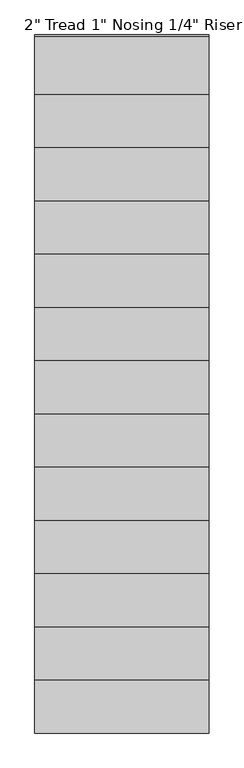
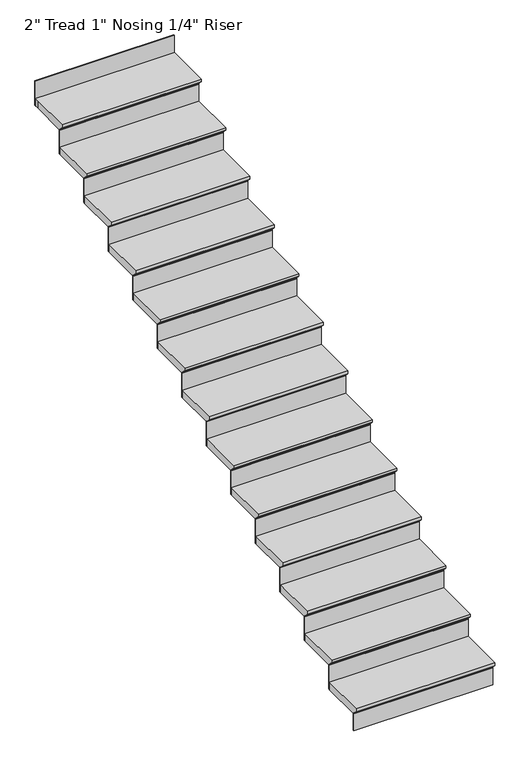
"""IFC4 building model written with IfcOpenShell, lengths in millimetres: stair flight geometry."""

from ifc_helpers import new_model, si_unit, origin, place, context, project, spatial, faceted_brep, source, transform, mapped, element, save


def stair_flight_ec606b3e(model_context):
    return source(origin(), model_context, "Body", "Brep", [
        faceted_brep([(-2703.0415084, -23154.3851539, 49768.9005799), (-2703.0415084, -23154.3851539, 49787.9505799), (-3617.4415084, -23154.3851539, 49787.9505799), (-3617.4415084, -23154.3851539, 49768.9005799), (-2703.0415084, -23128.9851539, 49743.5005799), (-3617.4415084, -23128.9851539, 49743.5005799), (-2703.0415084, -22849.5851539, 49787.9505799), (-3617.4415084, -22849.5851539, 49787.9505799), (-3617.4415084, -23128.9851539, 49737.1505799), (-3617.4415084, -22849.5851539, 49737.1505799), (-2703.0415084, -22849.5851539, 49737.1505799), (-2703.0415084, -23128.9851539, 49737.1505799)], [[[0, 1, 2, 3]], [[4, 0, 3, 5]], [[2, 1, 6, 7]], [[8, 9, 10, 11]], [[2, 7, 9, 8, 5, 3]], [[8, 11, 4, 5]], [[6, 1, 0, 4, 11, 10]], [[7, 6, 10, 9]]]),
        faceted_brep([(-2703.0415084, -23128.9851539, 49737.1505799), (-2703.0415084, -23128.9851539, 49618.6172466), (-2703.0415084, -23122.6351539, 49618.6172466), (-2703.0415084, -23122.6351539, 49737.1505799), (-3617.4415084, -23128.9851539, 49737.1505799), (-3617.4415084, -23122.6351539, 49737.1505799), (-3617.4415084, -23122.6351539, 49618.6172466), (-3617.4415084, -23128.9851539, 49618.6172466)], [[[0, 1, 2, 3]], [[4, 5, 6, 7]], [[1, 0, 4, 7]], [[2, 1, 7, 6]], [[3, 2, 6, 5]], [[0, 3, 5, 4]]]),
        faceted_brep([(-2703.0415084, -22849.5851539, 49906.4839133), (-2703.0415084, -22849.5851539, 49737.1505799), (-2703.0415084, -22843.2351539, 49737.1505799), (-2703.0415084, -22843.2351539, 49906.4839133), (-3617.4415084, -22849.5851539, 49906.4839133), (-3617.4415084, -22843.2351539, 49906.4839133), (-3617.4415084, -22843.2351539, 49737.1505799), (-3617.4415084, -22849.5851539, 49737.1505799)], [[[0, 1, 2, 3]], [[4, 5, 6, 7]], [[1, 0, 4, 7]], [[2, 1, 7, 6]], [[3, 2, 6, 5]], [[0, 3, 5, 4]]]),
        faceted_brep([(-3617.4415084, -22874.9851539, 49957.2839133), (-2703.0415084, -22874.9851539, 49957.2839133), (-2703.0415084, -22570.1851539, 49957.2839133), (-3617.4415084, -22570.1851539, 49957.2839133), (-3617.4415084, -22849.5851539, 49906.4839133), (-3617.4415084, -22570.1851539, 49906.4839133), (-2703.0415084, -22570.1851539, 49906.4839133), (-2703.0415084, -22849.5851539, 49906.4839133), (-3617.4415084, -22849.5851539, 49912.8339133), (-3617.4415084, -22874.9851539, 49938.2339133), (-2703.0415084, -22849.5851539, 49912.8339133), (-2703.0415084, -22874.9851539, 49938.2339133)], [[[0, 1, 2, 3]], [[4, 5, 6, 7]], [[0, 3, 5, 4, 8, 9]], [[4, 7, 10, 8]], [[2, 1, 11, 10, 7, 6]], [[3, 2, 6, 5]], [[11, 1, 0, 9]], [[10, 11, 9, 8]]]),
        faceted_brep([(-2703.0415084, -22570.1851539, 50075.8172466), (-2703.0415084, -22570.1851539, 49906.4839133), (-2703.0415084, -22563.8351539, 49906.4839133), (-2703.0415084, -22563.8351539, 50075.8172466), (-3617.4415084, -22570.1851539, 50075.8172466), (-3617.4415084, -22563.8351539, 50075.8172466), (-3617.4415084, -22563.8351539, 49906.4839133), (-3617.4415084, -22570.1851539, 49906.4839133)], [[[0, 1, 2, 3]], [[4, 5, 6, 7]], [[1, 0, 4, 7]], [[2, 1, 7, 6]], [[3, 2, 6, 5]], [[0, 3, 5, 4]]]),
        faceted_brep([(-3617.4415084, -22595.5851539, 50126.6172466), (-2703.0415084, -22595.5851539, 50126.6172466), (-2703.0415084, -22290.7851539, 50126.6172466), (-3617.4415084, -22290.7851539, 50126.6172466), (-3617.4415084, -22570.1851539, 50075.8172466), (-3617.4415084, -22290.7851539, 50075.8172466), (-2703.0415084, -22290.7851539, 50075.8172466), (-2703.0415084, -22570.1851539, 50075.8172466), (-3617.4415084, -22570.1851539, 50082.1672466), (-3617.4415084, -22595.5851539, 50107.5672466), (-2703.0415084, -22570.1851539, 50082.1672466), (-2703.0415084, -22595.5851539, 50107.5672466)], [[[0, 1, 2, 3]], [[4, 5, 6, 7]], [[0, 3, 5, 4, 8, 9]], [[4, 7, 10, 8]], [[2, 1, 11, 10, 7, 6]], [[3, 2, 6, 5]], [[11, 1, 0, 9]], [[10, 11, 9, 8]]]),
        faceted_brep([(-2703.0415084, -22290.7851539, 50245.1505799), (-2703.0415084, -22290.7851539, 50075.8172466), (-2703.0415084, -22284.4351539, 50075.8172466), (-2703.0415084, -22284.4351539, 50245.1505799), (-3617.4415084, -22290.7851539, 50245.1505799), (-3617.4415084, -22284.4351539, 50245.1505799), (-3617.4415084, -22284.4351539, 50075.8172466), (-3617.4415084, -22290.7851539, 50075.8172466)], [[[0, 1, 2, 3]], [[4, 5, 6, 7]], [[1, 0, 4, 7]], [[2, 1, 7, 6]], [[3, 2, 6, 5]], [[0, 3, 5, 4]]]),
        faceted_brep([(-3617.4415084, -22316.1851539, 50295.9505799), (-2703.0415084, -22316.1851539, 50295.9505799), (-2703.0415084, -22011.3851539, 50295.9505799), (-3617.4415084, -22011.3851539, 50295.9505799), (-3617.4415084, -22290.7851539, 50245.1505799), (-3617.4415084, -22011.3851539, 50245.1505799), (-2703.0415084, -22011.3851539, 50245.1505799), (-2703.0415084, -22290.7851539, 50245.1505799), (-3617.4415084, -22290.7851539, 50251.5005799), (-3617.4415084, -22316.1851539, 50276.9005799), (-2703.0415084, -22290.7851539, 50251.5005799), (-2703.0415084, -22316.1851539, 50276.9005799)], [[[0, 1, 2, 3]], [[4, 5, 6, 7]], [[0, 3, 5, 4, 8, 9]], [[4, 7, 10, 8]], [[2, 1, 11, 10, 7, 6]], [[3, 2, 6, 5]], [[11, 1, 0, 9]], [[10, 11, 9, 8]]]),
        faceted_brep([(-2703.0415084, -22011.3851539, 50414.4839133), (-2703.0415084, -22011.3851539, 50245.1505799), (-2703.0415084, -22005.0351539, 50245.1505799), (-2703.0415084, -22005.0351539, 50414.4839133), (-3617.4415084, -22011.3851539, 50414.4839133), (-3617.4415084, -22005.0351539, 50414.4839133), (-3617.4415084, -22005.0351539, 50245.1505799), (-3617.4415084, -22011.3851539, 50245.1505799)], [[[0, 1, 2, 3]], [[4, 5, 6, 7]], [[1, 0, 4, 7]], [[2, 1, 7, 6]], [[3, 2, 6, 5]], [[0, 3, 5, 4]]]),
        faceted_brep([(-3617.4415084, -22036.7851539, 50465.2839133), (-2703.0415084, -22036.7851539, 50465.2839133), (-2703.0415084, -21731.9851539, 50465.2839133), (-3617.4415084, -21731.9851539, 50465.2839133), (-3617.4415084, -22011.3851539, 50414.4839133), (-3617.4415084, -21731.9851539, 50414.4839133), (-2703.0415084, -21731.9851539, 50414.4839133), (-2703.0415084, -22011.3851539, 50414.4839133), (-3617.4415084, -22011.3851539, 50420.8339133), (-3617.4415084, -22036.7851539, 50446.2339133), (-2703.0415084, -22011.3851539, 50420.8339133), (-2703.0415084, -22036.7851539, 50446.2339133)], [[[0, 1, 2, 3]], [[4, 5, 6, 7]], [[0, 3, 5, 4, 8, 9]], [[4, 7, 10, 8]], [[2, 1, 11, 10, 7, 6]], [[3, 2, 6, 5]], [[11, 1, 0, 9]], [[10, 11, 9, 8]]]),
        faceted_brep([(-2703.0415084, -21731.9851539, 50583.8172466), (-2703.0415084, -21731.9851539, 50414.4839133), (-2703.0415084, -21725.6351539, 50414.4839133), (-2703.0415084, -21725.6351539, 50583.8172466), (-3617.4415084, -21731.9851539, 50583.8172466), (-3617.4415084, -21725.6351539, 50583.8172466), (-3617.4415084, -21725.6351539, 50414.4839133), (-3617.4415084, -21731.9851539, 50414.4839133)], [[[0, 1, 2, 3]], [[4, 5, 6, 7]], [[1, 0, 4, 7]], [[2, 1, 7, 6]], [[3, 2, 6, 5]], [[0, 3, 5, 4]]]),
        faceted_brep([(-3617.4415084, -21757.3851539, 50634.6172466), (-2703.0415084, -21757.3851539, 50634.6172466), (-2703.0415084, -21452.5851539, 50634.6172466), (-3617.4415084, -21452.5851539, 50634.6172466), (-3617.4415084, -21731.9851539, 50583.8172466), (-3617.4415084, -21452.5851539, 50583.8172466), (-2703.0415084, -21452.5851539, 50583.8172466), (-2703.0415084, -21731.9851539, 50583.8172466), (-3617.4415084, -21731.9851539, 50590.1672466), (-3617.4415084, -21757.3851539, 50615.5672466), (-2703.0415084, -21731.9851539, 50590.1672466), (-2703.0415084, -21757.3851539, 50615.5672466)], [[[0, 1, 2, 3]], [[4, 5, 6, 7]], [[0, 3, 5, 4, 8, 9]], [[4, 7, 10, 8]], [[2, 1, 11, 10, 7, 6]], [[3, 2, 6, 5]], [[11, 1, 0, 9]], [[10, 11, 9, 8]]]),
        faceted_brep([(-2703.0415084, -21452.5851539, 50753.1505799), (-2703.0415084, -21452.5851539, 50583.8172466), (-2703.0415084, -21446.2351539, 50583.8172466), (-2703.0415084, -21446.2351539, 50753.1505799), (-3617.4415084, -21452.5851539, 50753.1505799), (-3617.4415084, -21446.2351539, 50753.1505799), (-3617.4415084, -21446.2351539, 50583.8172466), (-3617.4415084, -21452.5851539, 50583.8172466)], [[[0, 1, 2, 3]], [[4, 5, 6, 7]], [[1, 0, 4, 7]], [[2, 1, 7, 6]], [[3, 2, 6, 5]], [[0, 3, 5, 4]]]),
        faceted_brep([(-3617.4415084, -21477.9851539, 50803.9505799), (-2703.0415084, -21477.9851539, 50803.9505799), (-2703.0415084, -21173.1851539, 50803.9505799), (-3617.4415084, -21173.1851539, 50803.9505799), (-3617.4415084, -21452.5851539, 50753.1505799), (-3617.4415084, -21173.1851539, 50753.1505799), (-2703.0415084, -21173.1851539, 50753.1505799), (-2703.0415084, -21452.5851539, 50753.1505799), (-3617.4415084, -21452.5851539, 50759.5005799), (-3617.4415084, -21477.9851539, 50784.9005799), (-2703.0415084, -21452.5851539, 50759.5005799), (-2703.0415084, -21477.9851539, 50784.9005799)], [[[0, 1, 2, 3]], [[4, 5, 6, 7]], [[0, 3, 5, 4, 8, 9]], [[4, 7, 10, 8]], [[2, 1, 11, 10, 7, 6]], [[3, 2, 6, 5]], [[11, 1, 0, 9]], [[10, 11, 9, 8]]]),
        faceted_brep([(-2703.0415084, -21173.1851539, 50922.4839133), (-2703.0415084, -21173.1851539, 50753.1505799), (-2703.0415084, -21166.8351539, 50753.1505799), (-2703.0415084, -21166.8351539, 50922.4839133), (-3617.4415084, -21173.1851539, 50922.4839133), (-3617.4415084, -21166.8351539, 50922.4839133), (-3617.4415084, -21166.8351539, 50753.1505799), (-3617.4415084, -21173.1851539, 50753.1505799)], [[[0, 1, 2, 3]], [[4, 5, 6, 7]], [[1, 0, 4, 7]], [[2, 1, 7, 6]], [[3, 2, 6, 5]], [[0, 3, 5, 4]]]),
        faceted_brep([(-3617.4415084, -21198.5851539, 50973.2839133), (-2703.0415084, -21198.5851539, 50973.2839133), (-2703.0415084, -20893.7851539, 50973.2839133), (-3617.4415084, -20893.7851539, 50973.2839133), (-3617.4415084, -21173.1851539, 50922.4839133), (-3617.4415084, -20893.7851539, 50922.4839133), (-2703.0415084, -20893.7851539, 50922.4839133), (-2703.0415084, -21173.1851539, 50922.4839133), (-3617.4415084, -21173.1851539, 50928.8339133), (-3617.4415084, -21198.5851539, 50954.2339133), (-2703.0415084, -21173.1851539, 50928.8339133), (-2703.0415084, -21198.5851539, 50954.2339133)], [[[0, 1, 2, 3]], [[4, 5, 6, 7]], [[0, 3, 5, 4, 8, 9]], [[4, 7, 10, 8]], [[2, 1, 11, 10, 7, 6]], [[3, 2, 6, 5]], [[11, 1, 0, 9]], [[10, 11, 9, 8]]]),
        faceted_brep([(-2703.0415084, -20893.7851539, 51091.8172466), (-2703.0415084, -20893.7851539, 50922.4839133), (-2703.0415084, -20887.4351539, 50922.4839133), (-2703.0415084, -20887.4351539, 51091.8172466), (-3617.4415084, -20893.7851539, 51091.8172466), (-3617.4415084, -20887.4351539, 51091.8172466), (-3617.4415084, -20887.4351539, 50922.4839133), (-3617.4415084, -20893.7851539, 50922.4839133)], [[[0, 1, 2, 3]], [[4, 5, 6, 7]], [[1, 0, 4, 7]], [[2, 1, 7, 6]], [[3, 2, 6, 5]], [[0, 3, 5, 4]]]),
        faceted_brep([(-3617.4415084, -20919.1851539, 51142.6172466), (-2703.0415084, -20919.1851539, 51142.6172466), (-2703.0415084, -20614.3851539, 51142.6172466), (-3617.4415084, -20614.3851539, 51142.6172466), (-3617.4415084, -20893.7851539, 51091.8172466), (-3617.4415084, -20614.3851539, 51091.8172466), (-2703.0415084, -20614.3851539, 51091.8172466), (-2703.0415084, -20893.7851539, 51091.8172466), (-3617.4415084, -20893.7851539, 51098.1672466), (-3617.4415084, -20919.1851539, 51123.5672466), (-2703.0415084, -20893.7851539, 51098.1672466), (-2703.0415084, -20919.1851539, 51123.5672466)], [[[0, 1, 2, 3]], [[4, 5, 6, 7]], [[0, 3, 5, 4, 8, 9]], [[4, 7, 10, 8]], [[2, 1, 11, 10, 7, 6]], [[3, 2, 6, 5]], [[11, 1, 0, 9]], [[10, 11, 9, 8]]]),
        faceted_brep([(-2703.0415084, -20614.3851539, 51261.1505799), (-2703.0415084, -20614.3851539, 51091.8172466), (-2703.0415084, -20608.0351539, 51091.8172466), (-2703.0415084, -20608.0351539, 51261.1505799), (-3617.4415084, -20614.3851539, 51261.1505799), (-3617.4415084, -20608.0351539, 51261.1505799), (-3617.4415084, -20608.0351539, 51091.8172466), (-3617.4415084, -20614.3851539, 51091.8172466)], [[[0, 1, 2, 3]], [[4, 5, 6, 7]], [[1, 0, 4, 7]], [[2, 1, 7, 6]], [[3, 2, 6, 5]], [[0, 3, 5, 4]]]),
        faceted_brep([(-3617.4415084, -20639.7851539, 51311.9505799), (-2703.0415084, -20639.7851539, 51311.9505799), (-2703.0415084, -20334.9851539, 51311.9505799), (-3617.4415084, -20334.9851539, 51311.9505799), (-3617.4415084, -20614.3851539, 51261.1505799), (-3617.4415084, -20334.9851539, 51261.1505799), (-2703.0415084, -20334.9851539, 51261.1505799), (-2703.0415084, -20614.3851539, 51261.1505799), (-3617.4415084, -20614.3851539, 51267.5005799), (-3617.4415084, -20639.7851539, 51292.9005799), (-2703.0415084, -20614.3851539, 51267.5005799), (-2703.0415084, -20639.7851539, 51292.9005799)], [[[0, 1, 2, 3]], [[4, 5, 6, 7]], [[0, 3, 5, 4, 8, 9]], [[4, 7, 10, 8]], [[2, 1, 11, 10, 7, 6]], [[3, 2, 6, 5]], [[11, 1, 0, 9]], [[10, 11, 9, 8]]]),
        faceted_brep([(-2703.0415084, -20334.9851539, 51430.4839133), (-2703.0415084, -20334.9851539, 51261.1505799), (-2703.0415084, -20328.6351539, 51261.1505799), (-2703.0415084, -20328.6351539, 51430.4839133), (-3617.4415084, -20334.9851539, 51430.4839133), (-3617.4415084, -20328.6351539, 51430.4839133), (-3617.4415084, -20328.6351539, 51261.1505799), (-3617.4415084, -20334.9851539, 51261.1505799)], [[[0, 1, 2, 3]], [[4, 5, 6, 7]], [[1, 0, 4, 7]], [[2, 1, 7, 6]], [[3, 2, 6, 5]], [[0, 3, 5, 4]]]),
        faceted_brep([(-3617.4415084, -20360.3851539, 51481.2839133), (-2703.0415084, -20360.3851539, 51481.2839133), (-2703.0415084, -20055.5851539, 51481.2839133), (-3617.4415084, -20055.5851539, 51481.2839133), (-3617.4415084, -20334.9851539, 51430.4839133), (-3617.4415084, -20055.5851539, 51430.4839133), (-2703.0415084, -20055.5851539, 51430.4839133), (-2703.0415084, -20334.9851539, 51430.4839133), (-3617.4415084, -20334.9851539, 51436.8339133), (-3617.4415084, -20360.3851539, 51462.2339133), (-2703.0415084, -20334.9851539, 51436.8339133), (-2703.0415084, -20360.3851539, 51462.2339133)], [[[0, 1, 2, 3]], [[4, 5, 6, 7]], [[0, 3, 5, 4, 8, 9]], [[4, 7, 10, 8]], [[2, 1, 11, 10, 7, 6]], [[3, 2, 6, 5]], [[11, 1, 0, 9]], [[10, 11, 9, 8]]]),
        faceted_brep([(-2703.0415084, -20055.5851539, 51599.8172466), (-2703.0415084, -20055.5851539, 51430.4839133), (-2703.0415084, -20049.2351539, 51430.4839133), (-2703.0415084, -20049.2351539, 51599.8172466), (-3617.4415084, -20055.5851539, 51599.8172466), (-3617.4415084, -20049.2351539, 51599.8172466), (-3617.4415084, -20049.2351539, 51430.4839133), (-3617.4415084, -20055.5851539, 51430.4839133)], [[[0, 1, 2, 3]], [[4, 5, 6, 7]], [[1, 0, 4, 7]], [[2, 1, 7, 6]], [[3, 2, 6, 5]], [[0, 3, 5, 4]]]),
        faceted_brep([(-3617.4415084, -20080.9851539, 51650.6172466), (-2703.0415084, -20080.9851539, 51650.6172466), (-2703.0415084, -19776.1851539, 51650.6172466), (-3617.4415084, -19776.1851539, 51650.6172466), (-3617.4415084, -20055.5851539, 51599.8172466), (-3617.4415084, -19776.1851539, 51599.8172466), (-2703.0415084, -19776.1851539, 51599.8172466), (-2703.0415084, -20055.5851539, 51599.8172466), (-3617.4415084, -20055.5851539, 51606.1672466), (-3617.4415084, -20080.9851539, 51631.5672466), (-2703.0415084, -20055.5851539, 51606.1672466), (-2703.0415084, -20080.9851539, 51631.5672466)], [[[0, 1, 2, 3]], [[4, 5, 6, 7]], [[0, 3, 5, 4, 8, 9]], [[4, 7, 10, 8]], [[2, 1, 11, 10, 7, 6]], [[3, 2, 6, 5]], [[11, 1, 0, 9]], [[10, 11, 9, 8]]]),
        faceted_brep([(-2703.0415084, -19496.7851539, 51938.4839133), (-2703.0415084, -19496.7851539, 51769.1505799), (-2703.0415084, -19490.4351539, 51769.1505799), (-2703.0415084, -19490.4351539, 51938.4839133), (-3617.4415084, -19496.7851539, 51938.4839133), (-3617.4415084, -19490.4351539, 51938.4839133), (-3617.4415084, -19490.4351539, 51769.1505799), (-3617.4415084, -19496.7851539, 51769.1505799)], [[[0, 1, 2, 3]], [[4, 5, 6, 7]], [[1, 0, 4, 7]], [[2, 1, 7, 6]], [[3, 2, 6, 5]], [[0, 3, 5, 4]]]),
        faceted_brep([(-2703.0415084, -19776.1851539, 51769.1505799), (-2703.0415084, -19776.1851539, 51599.8172466), (-2703.0415084, -19769.8351539, 51599.8172466), (-2703.0415084, -19769.8351539, 51769.1505799), (-3617.4415084, -19776.1851539, 51769.1505799), (-3617.4415084, -19769.8351539, 51769.1505799), (-3617.4415084, -19769.8351539, 51599.8172466), (-3617.4415084, -19776.1851539, 51599.8172466)], [[[0, 1, 2, 3]], [[4, 5, 6, 7]], [[1, 0, 4, 7]], [[2, 1, 7, 6]], [[3, 2, 6, 5]], [[0, 3, 5, 4]]]),
        faceted_brep([(-3617.4415084, -19496.7851539, 51819.9505799), (-3617.4415084, -19522.1851539, 51819.9505799), (-3617.4415084, -19801.5851539, 51819.9505799), (-2703.0415084, -19801.5851539, 51819.9505799), (-2703.0415084, -19496.7851539, 51819.9505799), (-3617.4415084, -19522.1851539, 51769.1505799), (-3617.4415084, -19496.7851539, 51769.1505799), (-2703.0415084, -19496.7851539, 51769.1505799), (-2703.0415084, -19776.1851539, 51769.1505799), (-3617.4415084, -19776.1851539, 51769.1505799), (-3617.4415084, -19776.1851539, 51775.5005799), (-3617.4415084, -19801.5851539, 51800.9005799), (-2703.0415084, -19776.1851539, 51775.5005799), (-2703.0415084, -19801.5851539, 51800.9005799)], [[[0, 1, 2, 3, 4]], [[5, 6, 7, 8, 9]], [[1, 0, 6, 5]], [[2, 1, 5, 9, 10, 11]], [[9, 8, 12, 10]], [[4, 3, 13, 12, 8, 7]], [[0, 4, 7, 6]], [[13, 3, 2, 11]], [[12, 13, 11, 10]]]),
    ])


if __name__ == "__main__":
    model = new_model("IFC4")
    model_context = context("Model", 3, world=origin())
    ifc_project = project(units=[si_unit("LENGTHUNIT", "METRE", prefix="MILLI")], contexts=[model_context])
    site = spatial("IfcSite", under=ifc_project)
    building = spatial("IfcBuilding", under=site)
    placement = place(None, origin())
    stair_flight_shape = stair_flight_ec606b3e(model_context)
    element("IfcStairFlight", 1, ObjectType="2\" Tread 1\" Nosing 1/4\" Riser", at=placement, inside=building, context=model_context, shape_type="MappedRepresentation", body=[
        mapped(stair_flight_shape, transform((0.0, 0.0, 0.0), x_axis=(1.0, 0.0, 0.0), y_axis=(0.0, 1.0, 0.0), z_axis=(0.0, 0.0, 1.0))),
    ])
    save(model, "model.ifc")
